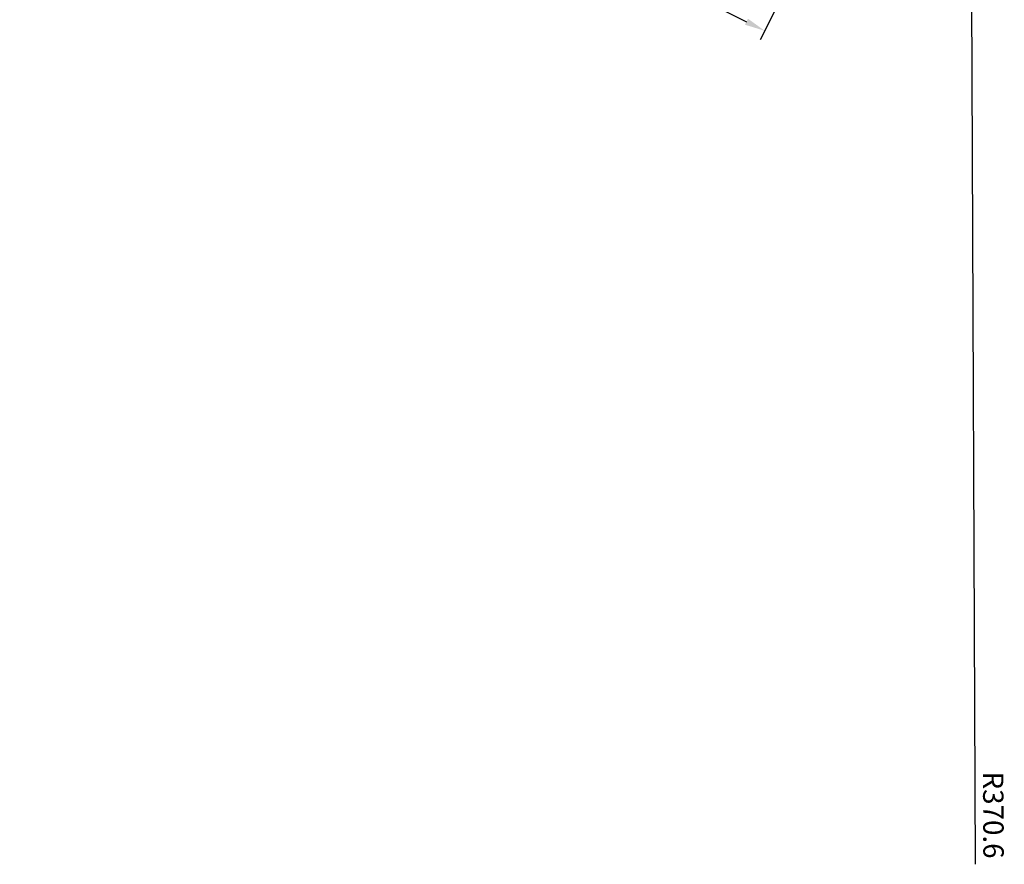
# Model space of a CAD drawing. Units: millimetres. Extents: x 1605 to 2079, y 1280 to 1879.
# Tile 1 of 7: x 1669 to 1790, y 1280 to 1384. Entities that reach past the tile are written whole.
import ezdxf

# ---------------------------------------------------------------- set-up
doc = ezdxf.new("R2010")
doc.units = ezdxf.units.MM
doc.layers.add('M-DIMS', color=2, linetype='Continuous', lineweight=25)
doc.styles.get("Standard").update_dxf_attribs({"font": 'arial.ttf'})
doc.dimstyles.new('ISO-25', dxfattribs={"dimtxt": 2.5, "dimasz": 2.5, "dimexe": 1.25, "dimexo": 0.625, "dimtad": 1, "dimdec": 0, "dimtxsty": 'Standard', "dimcen": 2.5, "dimadec": 0, "dimazin": 0, "dimtfac": 1, "dimtdec": 0, "dimtmove": 0, "dimatfit": 3, "dimfxl": 1, "dimarcsym": 0})

# ---------------------------------------------------------------- blocks, each defined once
blk = doc.blocks.new('*D24')
at = {"layer": 'Defpoints', "color": 0, "transparency": 16777216}
for p in [(1683.42, 1455.98), (1774.34, 1410.71), (1760.12, 1382.16)]:
    blk.add_point(p, dxfattribs=at)
at = {"layer": 'M-DIMS', "color": 0, "lineweight": -2, "transparency": 16777216}
for p, q in [((1683.14, 1455.42), (1668.64, 1426.31)), ((1671.44, 1426.31), (1757.89, 1383.27)), ((1774.06, 1410.15), (1759.57, 1381.04))]:
    blk.add_line(p, q, dxfattribs=at)
at = {"layer": 'M-DIMS', "color": 0, "transparency": 16777216}
for points in [[(1671.62, 1426.69), (1671.25, 1425.94), (1669.2, 1427.43)], [(1758.07, 1383.64), (1757.7, 1382.9), (1760.12, 1382.16)]]:
    blk.add_solid(points, dxfattribs=at)
at = {"layer": 'M-DIMS', "color": 0, "transparency": 16777216, "insert": (1715.51, 1406.5), "char_height": 2.5, "attachment_point": 5, "rotation": 333.531}
blk.add_mtext('102', dxfattribs=at)
blk = doc.blocks.new('*D71')
at = {"layer": 'Defpoints', "color": 0, "transparency": 16777216}
for p in [(1783.42, 1878.81), (1785.02, 1508.24)]:
    blk.add_point(p, dxfattribs=at)
at = {"layer": 'M-DIMS', "color": 0, "lineweight": -2, "transparency": 16777216}
for p, q in [((1783.42, 1878.81), (1785.02, 1508.24)), ((1786.01, 1279.86), (1785.03, 1505.74))]:
    blk.add_line(p, q, dxfattribs=at)
at = {"layer": 'M-DIMS', "color": 0, "transparency": 16777216}
blk.add_solid([(1785.45, 1505.74), (1784.61, 1505.73), (1785.02, 1508.24)], dxfattribs=at)
at = {"layer": 'M-DIMS', "color": 0, "transparency": 16777216, "insert": (1787.88, 1285.9), "char_height": 2.5, "attachment_point": 5, "rotation": 270.2478}
blk.add_mtext('R370.6', dxfattribs=at)

msp = doc.modelspace()

# ---------------------------------------------------------------- dimensions: what is measured, and where the dimension line sits
at = {"layer": 'M-DIMS'}
dim = msp.add_radius_dim(center=(1783.4159, 1878.8069), mpoint=(1785.0189, 1508.2365), dimstyle='ISO-25', override={"dimdec": 1, "dimlfac": 1, "dimrnd": 0, "dimzin": 0, "dimdsep": 46, "dimlunit": 2}, dxfattribs=at)
dim.commit()
dim.dimension.update_dxf_attribs({"geometry": '*D71', "text_midpoint": (1785.9807, 1285.8942), "dimtype": 164})
dim = msp.add_aligned_dim(p1=(1683.4159, 1455.9806), p2=(1774.3402, 1410.7088), distance=-31.8951, dimstyle='ISO-25', override={"dimclrd": 0, "dimclre": 0, "dimclrt": 0}, dxfattribs=at)
dim.commit()
dim.dimension.update_dxf_attribs({"geometry": '*D24', "text_midpoint": (1715.5095, 1406.4951)})

doc.saveas('drawing.dxf')
